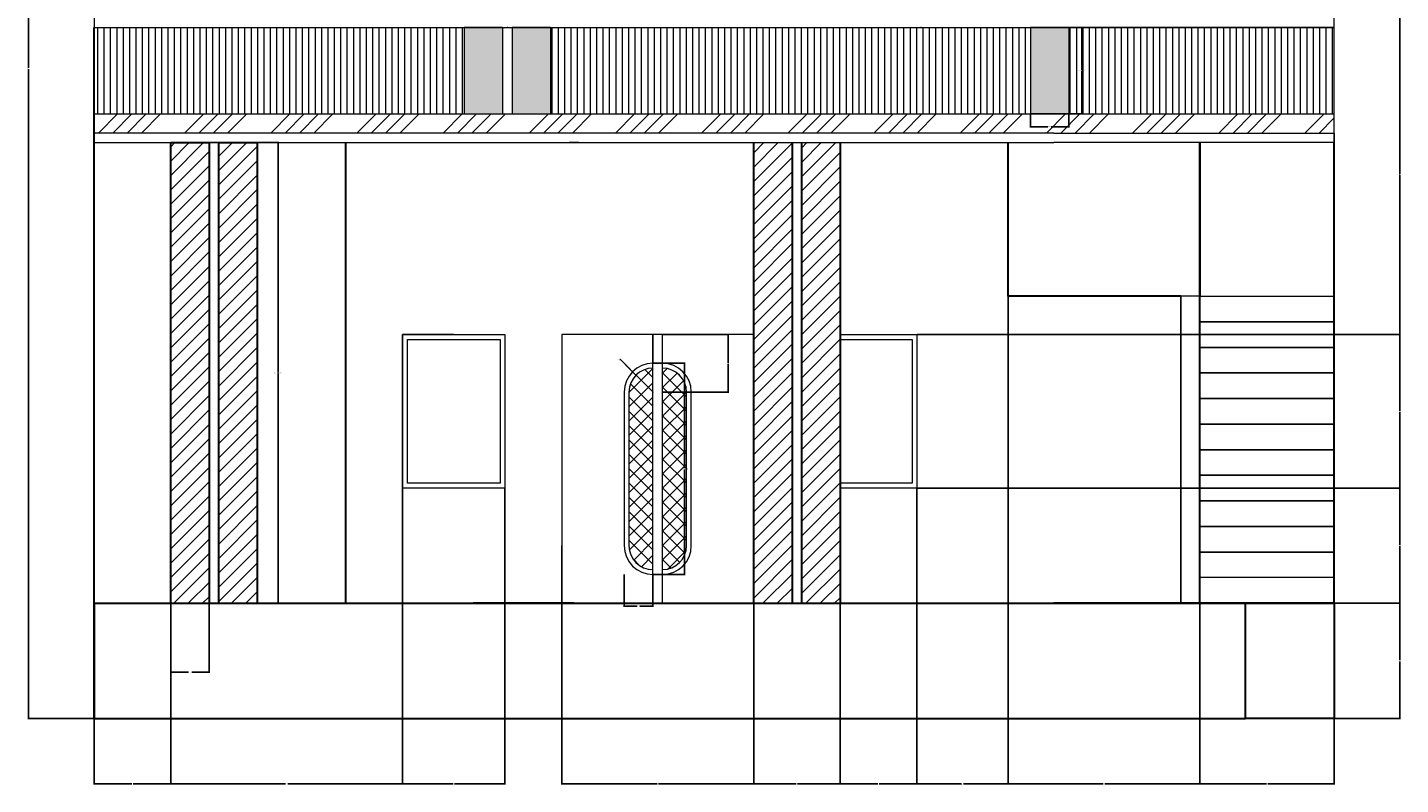
# Model space of a CAD drawing. Units: inches. Extents: x 2156 to 3149, y 1513 to 2286.
# Tile 4 of 5: x 2720 to 3149, y 1838 to 2075. Entities that reach past the tile are written whole.
import ezdxf

# ---------------------------------------------------------------- set-up
doc = ezdxf.new("R2010")
doc.units = ezdxf.units.IN
for name, color, linetype, lineweight in [('A-ANNO-DIMS', 2, 'Continuous', 18), ('A-CONS', 8, 'Continuous', 9), ('A-ELEV', 7, 'Continuous', 30), ('A-ELEV-BASE', 7, 'Continuous', 30), ('A-ELEV-COLS', 7, 'Continuous', 30), ('A-ELEV-COLS-PATT', 8, 'Continuous', 13), ('A-ELEV-DOOR', 3, 'Continuous', 20), ('A-ELEV-DOOR-PATT', 8, 'Continuous', 13), ('A-ELEV-GLAZ', 4, 'Continuous', 18), ('A-ELEV-PATT', 18, 'Continuous', 13), ('A-ELEV-STRS', 7, 'Continuous', 20), ('A-ELEV-TRIM', 7, 'Continuous', 20), ('A-ELEV-TRIM-PATT', 8, 'Continuous', 13)]:
    doc.layers.add(name, color=color, linetype=linetype, lineweight=lineweight)
doc.styles.get("Standard").update_dxf_attribs({"font": 'arial.ttf'})
doc.dimstyles.get("Standard").update_dxf_attribs({"dimtxt": 0.18, "dimasz": 0.18, "dimexe": 0.18, "dimexo": 0.0625, "dimgap": 0.09, "dimtad": 0, "dimtih": 1, "dimtoh": 1, "dimdec": 4, "dimzin": 0, "dimdsep": 46, "dimtxsty": 'Standard', "dimcen": 0.09, "dimadec": 0, "dimazin": 0, "dimtfac": 1, "dimtdec": 4, "dimtofl": 0, "dimtmove": 0, "dimatfit": 3, "dimfxl": 1, "dimtolj": 1, "dimtzin": 0, "dimarcsym": 0})

# ---------------------------------------------------------------- blocks, each defined once
blk = doc.blocks.new('ENTRY-DOOR-OVAL-TRIM')
for p, q in [((0, 57), (0, 9)), ((1.5, 57), (1.5, 9))]:
    blk.add_line(p, q)
for centre, radius, start, end in [((9, 57), 9, 90, 180), ((9, 57), 7.5, 90, 180), ((9, 9), 9, 180, 270), ((9, 9), 7.5, 180, 270)]:
    blk.add_arc(centre, radius, start, end)
blk = doc.blocks.new('FASCIA-PIER-12X27')
for p, q in [((12, 27), (0, 27)), ((0, 27), (0, 0)), ((12, 27), (12, 0))]:
    blk.add_line(p, q)
blk = doc.blocks.new('PORCH-PIER-12X144-ELEV')
for p, q in [((0, 0), (0, 144)), ((0, 144), (12, 144)), ((12, 144), (12, 0))]:
    blk.add_line(p, q)
blk = doc.blocks.new('*D13')
at = {"layer": 'A-ANNO-DIMS', "color": 0, "lineweight": -2, "transparency": 16777216}
for p, q in [((3045.59, 2074.71), (3049.76, 2074.71)), ((3049.58, 2074.53), (3049.58, 2061.39)), ((3049.58, 2047.89), (3049.58, 2061.03)), ((3045.59, 2047.71), (3049.76, 2047.71))]:
    blk.add_line(p, q, dxfattribs=at)
at = {"layer": 'A-ANNO-DIMS', "color": 0, "transparency": 16777216}
for points in [[(3049.55, 2074.53), (3049.61, 2074.53), (3049.58, 2074.71)], [(3049.55, 2047.89), (3049.61, 2047.89), (3049.58, 2047.71)]]:
    blk.add_solid(points, dxfattribs=at)
at = {"layer": 'Defpoints', "color": 0, "transparency": 16777216}
for p in [(3045.53, 2074.71), (3049.58, 2074.71), (3045.53, 2047.71)]:
    blk.add_point(p, dxfattribs=at)
at = {"layer": 'A-ANNO-DIMS', "color": 0, "transparency": 16777216, "insert": (3049.58, 2061.21), "char_height": 0.18, "attachment_point": 5}
blk.add_mtext('\\A1;FASCIA PIER 27 TYP.', dxfattribs=at)
blk = doc.blocks.new('*D14')
at = {"layer": 'A-ANNO-DIMS', "color": 0, "lineweight": -2, "transparency": 16777216}
for p, q in [((3033.53, 2047.65), (3033.53, 2043.48)), ((3045.53, 2047.65), (3045.53, 2043.48)), ((3033.71, 2043.66), (3039.01, 2043.66)), ((3045.35, 2043.66), (3040.05, 2043.66))]:
    blk.add_line(p, q, dxfattribs=at)
at = {"layer": 'A-ANNO-DIMS', "color": 0, "transparency": 16777216}
for points in [[(3033.71, 2043.69), (3033.71, 2043.63), (3033.53, 2043.66)], [(3045.35, 2043.69), (3045.35, 2043.63), (3045.53, 2043.66)]]:
    blk.add_solid(points, dxfattribs=at)
at = {"layer": 'Defpoints', "color": 0, "transparency": 16777216}
for p in [(3033.53, 2047.71), (3045.53, 2047.71), (3045.53, 2043.66)]:
    blk.add_point(p, dxfattribs=at)
at = {"layer": 'A-ANNO-DIMS', "color": 0, "transparency": 16777216, "insert": (3039.53, 2043.66), "char_height": 0.18, "attachment_point": 5}
blk.add_mtext('\\A1;12 TYP.', dxfattribs=at)
blk = doc.blocks.new('*D15')
at = {"layer": 'A-ANNO-DIMS', "color": 0, "lineweight": -2, "transparency": 16777216}
for p, q in [((2915.59, 1969.71), (2925.61, 1969.71)), ((2925.43, 1969.53), (2925.43, 1936.89)), ((2925.43, 1903.89), (2925.43, 1936.53)), ((2915.59, 1903.71), (2925.61, 1903.71))]:
    blk.add_line(p, q, dxfattribs=at)
at = {"layer": 'A-ANNO-DIMS', "color": 0, "transparency": 16777216}
for points in [[(2925.4, 1969.53), (2925.46, 1969.53), (2925.43, 1969.71)], [(2925.4, 1903.89), (2925.46, 1903.89), (2925.43, 1903.71)]]:
    blk.add_solid(points, dxfattribs=at)
at = {"layer": 'Defpoints', "color": 0, "transparency": 16777216}
for p in [(2915.53, 1969.71), (2925.43, 1969.71), (2915.53, 1903.71)]:
    blk.add_point(p, dxfattribs=at)
at = {"layer": 'A-ANNO-DIMS', "color": 0, "transparency": 16777216, "insert": (2925.43, 1936.71), "char_height": 0.18, "attachment_point": 5}
blk.add_mtext('\\A1;DOOR TRIM 66 TYP.', dxfattribs=at)
blk = doc.blocks.new('*D16')
at = {"layer": 'A-ANNO-DIMS', "color": 0, "lineweight": -2, "transparency": 16777216}
for p, q in [((2906.53, 1903.65), (2906.53, 1893.63)), ((2915.53, 1903.65), (2915.53, 1893.63)), ((2906.71, 1893.81), (2910.57, 1893.81)), ((2915.35, 1893.81), (2911.48, 1893.81))]:
    blk.add_line(p, q, dxfattribs=at)
at = {"layer": 'A-ANNO-DIMS', "color": 0, "transparency": 16777216}
for points in [[(2906.71, 1893.84), (2906.71, 1893.78), (2906.53, 1893.81)], [(2915.35, 1893.84), (2915.35, 1893.78), (2915.53, 1893.81)]]:
    blk.add_solid(points, dxfattribs=at)
at = {"layer": 'Defpoints', "color": 0, "transparency": 16777216}
for p in [(2906.53, 1903.71), (2915.53, 1903.71), (2915.53, 1893.81)]:
    blk.add_point(p, dxfattribs=at)
at = {"layer": 'A-ANNO-DIMS', "color": 0, "transparency": 16777216, "insert": (2911.03, 1893.81), "char_height": 0.18, "attachment_point": 5}
blk.add_mtext('\\A1;9 TYP.', dxfattribs=at)
blk = doc.blocks.new('*D17')
at = {"layer": 'A-ANNO-DIMS', "color": 0, "lineweight": -2, "transparency": 16777216}
for p, q in [((2776.88, 2038.71), (2798.6, 2038.71)), ((2798.42, 2038.53), (2798.42, 1966.89)), ((2798.42, 1894.89), (2798.42, 1966.53)), ((2776.88, 1894.71), (2798.6, 1894.71))]:
    blk.add_line(p, q, dxfattribs=at)
at = {"layer": 'A-ANNO-DIMS', "color": 0, "transparency": 16777216}
for points in [[(2798.39, 2038.53), (2798.45, 2038.53), (2798.42, 2038.71)], [(2798.39, 1894.89), (2798.45, 1894.89), (2798.42, 1894.71)]]:
    blk.add_solid(points, dxfattribs=at)
at = {"layer": 'Defpoints', "color": 0, "transparency": 16777216}
for p in [(2776.82, 2038.71), (2798.42, 2038.71), (2776.82, 1894.71)]:
    blk.add_point(p, dxfattribs=at)
at = {"layer": 'A-ANNO-DIMS', "color": 0, "transparency": 16777216, "insert": (2798.42, 1966.71), "char_height": 0.18, "attachment_point": 5}
blk.add_mtext('\\A1;PORCH PIER 144 TYP.', dxfattribs=at)
blk = doc.blocks.new('*D18')
at = {"layer": 'A-ANNO-DIMS', "color": 0, "lineweight": -2, "transparency": 16777216}
for p, q in [((2764.82, 1894.65), (2764.82, 1872.93)), ((2776.82, 1894.65), (2776.82, 1872.93)), ((2765, 1873.11), (2770.3, 1873.11)), ((2776.64, 1873.11), (2771.34, 1873.11))]:
    blk.add_line(p, q, dxfattribs=at)
at = {"layer": 'A-ANNO-DIMS', "color": 0, "transparency": 16777216}
for points in [[(2765, 1873.14), (2765, 1873.08), (2764.82, 1873.11)], [(2776.64, 1873.14), (2776.64, 1873.08), (2776.82, 1873.11)]]:
    blk.add_solid(points, dxfattribs=at)
at = {"layer": 'Defpoints', "color": 0, "transparency": 16777216}
for p in [(2764.82, 1894.71), (2776.82, 1894.71), (2776.82, 1873.11)]:
    blk.add_point(p, dxfattribs=at)
at = {"layer": 'A-ANNO-DIMS', "color": 0, "transparency": 16777216, "insert": (2770.82, 1873.11), "char_height": 0.18, "attachment_point": 5}
blk.add_mtext('\\A1;12 TYP.', dxfattribs=at)
blk = doc.blocks.new('*D46')
at = {"layer": 'A-ANNO-DIMS', "color": 0, "lineweight": -2, "transparency": 16777216}
for p, q in [((3071.46, 2265.09), (2720.14, 2265.09)), ((2720.32, 2264.91), (2720.32, 2062.08)), ((2720.32, 1858.89), (2720.32, 2061.72)), ((2740.75, 1858.71), (2720.14, 1858.71))]:
    blk.add_line(p, q, dxfattribs=at)
at = {"layer": 'A-ANNO-DIMS', "color": 0, "transparency": 16777216}
for points in [[(2720.29, 2264.91), (2720.35, 2264.91), (2720.32, 2265.09)], [(2720.29, 1858.89), (2720.35, 1858.89), (2720.32, 1858.71)]]:
    blk.add_solid(points, dxfattribs=at)
at = {"layer": 'Defpoints', "color": 0, "transparency": 16777216}
for p in [(2720.32, 2265.09), (3071.53, 2265.09), (2740.82, 1858.71)]:
    blk.add_point(p, dxfattribs=at)
at = {"layer": 'A-ANNO-DIMS', "color": 0, "transparency": 16777216, "insert": (2720.32, 2061.9), "char_height": 0.18, "attachment_point": 5}
blk.add_mtext('\\A1;406.4', dxfattribs=at)
blk = doc.blocks.new('*D48')
at = {"layer": 'A-ANNO-DIMS', "color": 0, "lineweight": -2, "transparency": 16777216}
for p, q in [((2918.59, 1978.71), (2939.21, 1978.71)), ((2939.03, 1978.53), (2939.03, 1969.89)), ((2939.03, 1960.89), (2939.03, 1969.53)), ((2918.59, 1960.71), (2939.21, 1960.71))]:
    blk.add_line(p, q, dxfattribs=at)
at = {"layer": 'A-ANNO-DIMS', "color": 0, "transparency": 16777216}
for points in [[(2939, 1978.53), (2939.06, 1978.53), (2939.03, 1978.71)], [(2939, 1960.89), (2939.06, 1960.89), (2939.03, 1960.71)]]:
    blk.add_solid(points, dxfattribs=at)
at = {"layer": 'Defpoints', "color": 0, "transparency": 16777216}
for p in [(2918.53, 1978.71), (2918.53, 1960.71), (2939.03, 1960.71)]:
    blk.add_point(p, dxfattribs=at)
at = {"layer": 'A-ANNO-DIMS', "color": 0, "transparency": 16777216, "insert": (2939.03, 1969.71), "char_height": 0.18, "attachment_point": 5}
blk.add_mtext('\\A1;18', dxfattribs=at)
blk = doc.blocks.new('*D51')
at = {"layer": 'A-ANNO-DIMS', "color": 0, "lineweight": -2, "transparency": 16777216}
for p, q in [((3128.59, 1894.71), (3149.21, 1894.71)), ((3149.03, 1894.53), (3149.03, 1876.89)), ((3149.03, 1858.89), (3149.03, 1876.53)), ((3128.59, 1858.71), (3149.21, 1858.71))]:
    blk.add_line(p, q, dxfattribs=at)
at = {"layer": 'A-ANNO-DIMS', "color": 0, "transparency": 16777216}
for points in [[(3149, 1894.53), (3149.06, 1894.53), (3149.03, 1894.71)], [(3149, 1858.89), (3149.06, 1858.89), (3149.03, 1858.71)]]:
    blk.add_solid(points, dxfattribs=at)
at = {"layer": 'Defpoints', "color": 0, "transparency": 16777216}
for p in [(3128.53, 1894.71), (3149.03, 1894.71), (3128.53, 1858.71)]:
    blk.add_point(p, dxfattribs=at)
at = {"layer": 'A-ANNO-DIMS', "color": 0, "transparency": 16777216, "insert": (3149.03, 1876.71), "char_height": 0.18, "attachment_point": 5}
blk.add_mtext('\\A1;36', dxfattribs=at)
blk = doc.blocks.new('*D52')
at = {"layer": 'A-ANNO-DIMS', "color": 0, "lineweight": -2, "transparency": 16777216}
for p, q in [((2998.09, 1930.71), (3149.21, 1930.71)), ((3149.03, 1930.53), (3149.03, 1912.89)), ((3149.03, 1894.89), (3149.03, 1912.53)), ((3128.59, 1894.71), (3149.21, 1894.71))]:
    blk.add_line(p, q, dxfattribs=at)
at = {"layer": 'A-ANNO-DIMS', "color": 0, "transparency": 16777216}
for points in [[(3149, 1930.53), (3149.06, 1930.53), (3149.03, 1930.71)], [(3149, 1894.89), (3149.06, 1894.89), (3149.03, 1894.71)]]:
    blk.add_solid(points, dxfattribs=at)
at = {"layer": 'Defpoints', "color": 0, "transparency": 16777216}
for p in [(2998.03, 1930.71), (3149.03, 1930.71), (3128.53, 1894.71)]:
    blk.add_point(p, dxfattribs=at)
at = {"layer": 'A-ANNO-DIMS', "color": 0, "transparency": 16777216, "insert": (3149.03, 1912.71), "char_height": 0.18, "attachment_point": 5}
blk.add_mtext('\\A1;36', dxfattribs=at)
blk = doc.blocks.new('*D53')
at = {"layer": 'A-ANNO-DIMS', "color": 0, "lineweight": -2, "transparency": 16777216}
for p, q in [((2998.09, 1978.71), (3149.21, 1978.71)), ((3149.03, 1978.53), (3149.03, 1954.89)), ((3149.03, 1930.89), (3149.03, 1954.53)), ((2998.09, 1930.71), (3149.21, 1930.71))]:
    blk.add_line(p, q, dxfattribs=at)
at = {"layer": 'A-ANNO-DIMS', "color": 0, "transparency": 16777216}
for points in [[(3149, 1978.53), (3149.06, 1978.53), (3149.03, 1978.71)], [(3149, 1930.89), (3149.06, 1930.89), (3149.03, 1930.71)]]:
    blk.add_solid(points, dxfattribs=at)
at = {"layer": 'Defpoints', "color": 0, "transparency": 16777216}
for p in [(2998.03, 1978.71), (3149.03, 1978.71), (2998.03, 1930.71)]:
    blk.add_point(p, dxfattribs=at)
at = {"layer": 'A-ANNO-DIMS', "color": 0, "transparency": 16777216, "insert": (3149.03, 1954.71), "char_height": 0.18, "attachment_point": 5}
blk.add_mtext('\\A1;48', dxfattribs=at)
blk = doc.blocks.new('*D54')
at = {"layer": 'A-ANNO-DIMS', "color": 0, "lineweight": -2, "transparency": 16777216}
for p, q in [((3128.59, 2078.71), (3149.21, 2078.71)), ((3149.03, 2078.53), (3149.03, 2028.89)), ((3149.03, 1978.89), (3149.03, 2028.53)), ((2998.09, 1978.71), (3149.21, 1978.71))]:
    blk.add_line(p, q, dxfattribs=at)
at = {"layer": 'A-ANNO-DIMS', "color": 0, "transparency": 16777216}
for points in [[(3149, 2078.53), (3149.06, 2078.53), (3149.03, 2078.71)], [(3149, 1978.89), (3149.06, 1978.89), (3149.03, 1978.71)]]:
    blk.add_solid(points, dxfattribs=at)
at = {"layer": 'Defpoints', "color": 0, "transparency": 16777216}
for p in [(3128.53, 2078.71), (3149.03, 2078.71), (2998.03, 1978.71)]:
    blk.add_point(p, dxfattribs=at)
at = {"layer": 'A-ANNO-DIMS', "color": 0, "transparency": 16777216, "insert": (3149.03, 2028.71), "char_height": 0.18, "attachment_point": 5}
blk.add_mtext('\\A1;100', dxfattribs=at)
blk = doc.blocks.new('*D58')
at = {"layer": 'A-ANNO-DIMS', "color": 0, "lineweight": -2, "transparency": 16777216}
for p, q in [((2764.82, 1894.65), (2764.82, 1838.03)), ((2740.82, 1858.65), (2740.82, 1838.03)), ((2741, 1838.21), (2752.6, 1838.21)), ((2764.64, 1838.21), (2753.04, 1838.21))]:
    blk.add_line(p, q, dxfattribs=at)
at = {"layer": 'A-ANNO-DIMS', "color": 0, "transparency": 16777216}
for points in [[(2741, 1838.24), (2741, 1838.18), (2740.82, 1838.21)], [(2764.64, 1838.24), (2764.64, 1838.18), (2764.82, 1838.21)]]:
    blk.add_solid(points, dxfattribs=at)
at = {"layer": 'Defpoints', "color": 0, "transparency": 16777216}
for p in [(2764.82, 1894.71), (2740.82, 1858.71), (2764.82, 1838.21)]:
    blk.add_point(p, dxfattribs=at)
at = {"layer": 'A-ANNO-DIMS', "color": 0, "transparency": 16777216, "insert": (2752.82, 1838.21), "char_height": 0.18, "attachment_point": 5}
blk.add_mtext('\\A1;24', dxfattribs=at)
blk = doc.blocks.new('*D59')
at = {"layer": 'A-ANNO-DIMS', "color": 0, "lineweight": -2, "transparency": 16777216}
for p, q in [((2837.28, 1930.65), (2837.28, 1838.03)), ((2764.82, 1894.65), (2764.82, 1838.03)), ((2765, 1838.21), (2800.65, 1838.21)), ((2837.1, 1838.21), (2801.44, 1838.21))]:
    blk.add_line(p, q, dxfattribs=at)
at = {"layer": 'A-ANNO-DIMS', "color": 0, "transparency": 16777216}
for points in [[(2765, 1838.24), (2765, 1838.18), (2764.82, 1838.21)], [(2837.1, 1838.24), (2837.1, 1838.18), (2837.28, 1838.21)]]:
    blk.add_solid(points, dxfattribs=at)
at = {"layer": 'Defpoints', "color": 0, "transparency": 16777216}
for p in [(2837.28, 1930.71), (2764.82, 1894.71), (2837.28, 1838.21)]:
    blk.add_point(p, dxfattribs=at)
at = {"layer": 'A-ANNO-DIMS', "color": 0, "transparency": 16777216, "insert": (2801.05, 1838.21), "char_height": 0.18, "attachment_point": 5}
blk.add_mtext('\\A1;72.46', dxfattribs=at)
blk = doc.blocks.new('*D60')
at = {"layer": 'A-ANNO-DIMS', "color": 0, "lineweight": -2, "transparency": 16777216}
for p, q in [((2837.28, 1930.65), (2837.28, 1838.03)), ((2869.28, 1930.65), (2869.28, 1838.03)), ((2837.46, 1838.21), (2853.06, 1838.21)), ((2869.1, 1838.21), (2853.49, 1838.21))]:
    blk.add_line(p, q, dxfattribs=at)
at = {"layer": 'A-ANNO-DIMS', "color": 0, "transparency": 16777216}
for points in [[(2837.46, 1838.24), (2837.46, 1838.18), (2837.28, 1838.21)], [(2869.1, 1838.24), (2869.1, 1838.18), (2869.28, 1838.21)]]:
    blk.add_solid(points, dxfattribs=at)
at = {"layer": 'Defpoints', "color": 0, "transparency": 16777216}
for p in [(2837.28, 1930.71), (2869.28, 1930.71), (2869.28, 1838.21)]:
    blk.add_point(p, dxfattribs=at)
at = {"layer": 'A-ANNO-DIMS', "color": 0, "transparency": 16777216, "insert": (2853.28, 1838.21), "char_height": 0.18, "attachment_point": 5}
blk.add_mtext('\\A1;32', dxfattribs=at)
blk = doc.blocks.new('*D61')
at = {"layer": 'A-ANNO-DIMS', "color": 0, "lineweight": -2, "transparency": 16777216}
for p, q in [((2887.03, 1894.65), (2887.03, 1838.03)), ((2947.03, 1894.65), (2947.03, 1838.03)), ((2887.21, 1838.21), (2916.81, 1838.21)), ((2946.85, 1838.21), (2917.25, 1838.21))]:
    blk.add_line(p, q, dxfattribs=at)
at = {"layer": 'A-ANNO-DIMS', "color": 0, "transparency": 16777216}
for points in [[(2887.21, 1838.24), (2887.21, 1838.18), (2887.03, 1838.21)], [(2946.85, 1838.24), (2946.85, 1838.18), (2947.03, 1838.21)]]:
    blk.add_solid(points, dxfattribs=at)
at = {"layer": 'Defpoints', "color": 0, "transparency": 16777216}
for p in [(2887.03, 1894.71), (2947.03, 1894.71), (2947.03, 1838.21)]:
    blk.add_point(p, dxfattribs=at)
at = {"layer": 'A-ANNO-DIMS', "color": 0, "transparency": 16777216, "insert": (2917.03, 1838.21), "char_height": 0.18, "attachment_point": 5}
blk.add_mtext('\\A1;60', dxfattribs=at)
blk = doc.blocks.new('*D62')
at = {"layer": 'A-ANNO-DIMS', "color": 0, "lineweight": -2, "transparency": 16777216}
for p, q in [((2974.03, 1930.65), (2974.03, 1838.03)), ((2947.03, 1894.65), (2947.03, 1838.03)), ((2947.21, 1838.21), (2960.31, 1838.21)), ((2973.85, 1838.21), (2960.75, 1838.21))]:
    blk.add_line(p, q, dxfattribs=at)
at = {"layer": 'A-ANNO-DIMS', "color": 0, "transparency": 16777216}
for points in [[(2947.21, 1838.24), (2947.21, 1838.18), (2947.03, 1838.21)], [(2973.85, 1838.24), (2973.85, 1838.18), (2974.03, 1838.21)]]:
    blk.add_solid(points, dxfattribs=at)
at = {"layer": 'Defpoints', "color": 0, "transparency": 16777216}
for p in [(2974.03, 1930.71), (2947.03, 1894.71), (2974.03, 1838.21)]:
    blk.add_point(p, dxfattribs=at)
at = {"layer": 'A-ANNO-DIMS', "color": 0, "transparency": 16777216, "insert": (2960.53, 1838.21), "char_height": 0.18, "attachment_point": 5}
blk.add_mtext('\\A1;27', dxfattribs=at)
blk = doc.blocks.new('*D63')
at = {"layer": 'A-ANNO-DIMS', "color": 0, "lineweight": -2, "transparency": 16777216}
for p, q in [((2974.03, 1930.65), (2974.03, 1838.03)), ((2998.03, 1930.65), (2998.03, 1838.03)), ((2974.21, 1838.21), (2985.81, 1838.21)), ((2997.85, 1838.21), (2986.25, 1838.21))]:
    blk.add_line(p, q, dxfattribs=at)
at = {"layer": 'A-ANNO-DIMS', "color": 0, "transparency": 16777216}
for points in [[(2974.21, 1838.24), (2974.21, 1838.18), (2974.03, 1838.21)], [(2997.85, 1838.24), (2997.85, 1838.18), (2998.03, 1838.21)]]:
    blk.add_solid(points, dxfattribs=at)
at = {"layer": 'Defpoints', "color": 0, "transparency": 16777216}
for p in [(2974.03, 1930.71), (2998.03, 1930.71), (2998.03, 1838.21)]:
    blk.add_point(p, dxfattribs=at)
at = {"layer": 'A-ANNO-DIMS', "color": 0, "transparency": 16777216, "insert": (2986.03, 1838.21), "char_height": 0.18, "attachment_point": 5}
blk.add_mtext('\\A1;24', dxfattribs=at)
blk = doc.blocks.new('*D64')
at = {"layer": 'A-ANNO-DIMS', "color": 0, "lineweight": -2, "transparency": 16777216}
for p, q in [((3026.53, 1990.65), (3026.53, 1838.03)), ((2998.03, 1930.65), (2998.03, 1838.03)), ((2998.21, 1838.21), (3011.95, 1838.21)), ((3026.35, 1838.21), (3012.6, 1838.21))]:
    blk.add_line(p, q, dxfattribs=at)
at = {"layer": 'A-ANNO-DIMS', "color": 0, "transparency": 16777216}
for points in [[(2998.21, 1838.24), (2998.21, 1838.18), (2998.03, 1838.21)], [(3026.35, 1838.24), (3026.35, 1838.18), (3026.53, 1838.21)]]:
    blk.add_solid(points, dxfattribs=at)
at = {"layer": 'Defpoints', "color": 0, "transparency": 16777216}
for p in [(3026.53, 1990.71), (2998.03, 1930.71), (3026.53, 1838.21)]:
    blk.add_point(p, dxfattribs=at)
at = {"layer": 'A-ANNO-DIMS', "color": 0, "transparency": 16777216, "insert": (3012.28, 1838.21), "char_height": 0.18, "attachment_point": 5}
blk.add_mtext('\\A1;28.5', dxfattribs=at)
blk = doc.blocks.new('*D65')
at = {"layer": 'A-ANNO-DIMS', "color": 0, "lineweight": -2, "transparency": 16777216}
for p, q in [((3026.53, 1990.65), (3026.53, 1838.03)), ((3086.53, 1894.65), (3086.53, 1838.03)), ((3026.71, 1838.21), (3056.31, 1838.21)), ((3086.35, 1838.21), (3056.75, 1838.21))]:
    blk.add_line(p, q, dxfattribs=at)
at = {"layer": 'A-ANNO-DIMS', "color": 0, "transparency": 16777216}
for points in [[(3026.71, 1838.24), (3026.71, 1838.18), (3026.53, 1838.21)], [(3086.35, 1838.24), (3086.35, 1838.18), (3086.53, 1838.21)]]:
    blk.add_solid(points, dxfattribs=at)
at = {"layer": 'Defpoints', "color": 0, "transparency": 16777216}
for p in [(3026.53, 1990.71), (3086.53, 1894.71), (3086.53, 1838.21)]:
    blk.add_point(p, dxfattribs=at)
at = {"layer": 'A-ANNO-DIMS', "color": 0, "transparency": 16777216, "insert": (3056.53, 1838.21), "char_height": 0.18, "attachment_point": 5}
blk.add_mtext('\\A1;60', dxfattribs=at)
blk = doc.blocks.new('*D66')
at = {"layer": 'A-ANNO-DIMS', "color": 0, "lineweight": -2, "transparency": 16777216}
for p, q in [((3086.53, 1894.65), (3086.53, 1838.03)), ((3128.53, 1858.65), (3128.53, 1838.03)), ((3086.71, 1838.21), (3107.3, 1838.21)), ((3128.35, 1838.21), (3107.75, 1838.21))]:
    blk.add_line(p, q, dxfattribs=at)
at = {"layer": 'A-ANNO-DIMS', "color": 0, "transparency": 16777216}
for points in [[(3086.71, 1838.24), (3086.71, 1838.18), (3086.53, 1838.21)], [(3128.35, 1838.24), (3128.35, 1838.18), (3128.53, 1838.21)]]:
    blk.add_solid(points, dxfattribs=at)
at = {"layer": 'Defpoints', "color": 0, "transparency": 16777216}
for p in [(3086.53, 1894.71), (3128.53, 1858.71), (3128.53, 1838.21)]:
    blk.add_point(p, dxfattribs=at)
at = {"layer": 'A-ANNO-DIMS', "color": 0, "transparency": 16777216, "insert": (3107.53, 1838.21), "char_height": 0.18, "attachment_point": 5}
blk.add_mtext('\\A1;42', dxfattribs=at)
blk = doc.blocks.new('*D88')
at = {"layer": 'A-ANNO-DIMS', "color": 0, "lineweight": -2, "transparency": 16777216}
for p, q in [((2905.16, 1970.89), (2905.34, 1970.89)), ((2905.34, 1970.89), (2909.03, 1967.2)), ((2915.44, 1960.71), (2915.62, 1960.71)), ((2915.53, 1960.62), (2915.53, 1960.8))]:
    blk.add_line(p, q, dxfattribs=at)
at = {"layer": 'A-ANNO-DIMS', "color": 0, "transparency": 16777216}
blk.add_solid([(2909.06, 1967.22), (2909.01, 1967.18), (2909.16, 1967.07)], dxfattribs=at)
at = {"layer": 'Defpoints', "color": 0, "transparency": 16777216}
for p in [(2909.16, 1967.07), (2915.53, 1960.71)]:
    blk.add_point(p, dxfattribs=at)
at = {"layer": 'A-ANNO-DIMS', "color": 0, "transparency": 16777216, "insert": (2904.73, 1970.89), "char_height": 0.18, "attachment_point": 5}
blk.add_mtext('\\A1;4X R9', dxfattribs=at)
blk = doc.blocks.new('*D89')
at = {"layer": 'A-ANNO-DIMS', "color": 0, "lineweight": -2, "transparency": 16777216}
for p, q in [((2906.86, 1969.19), (2907.04, 1969.19)), ((2907.04, 1969.19), (2910.1, 1966.14)), ((2915.44, 1960.71), (2915.62, 1960.71)), ((2915.53, 1960.62), (2915.53, 1960.8))]:
    blk.add_line(p, q, dxfattribs=at)
at = {"layer": 'A-ANNO-DIMS', "color": 0, "transparency": 16777216}
blk.add_solid([(2910.12, 1966.16), (2910.07, 1966.12), (2910.22, 1966.01)], dxfattribs=at)
at = {"layer": 'Defpoints', "color": 0, "transparency": 16777216}
for p in [(2910.22, 1966.01), (2915.53, 1960.71)]:
    blk.add_point(p, dxfattribs=at)
at = {"layer": 'A-ANNO-DIMS', "color": 0, "transparency": 16777216, "insert": (2906.32, 1969.19), "char_height": 0.18, "attachment_point": 5}
blk.add_mtext('\\A1;4X R7.5', dxfattribs=at)

msp = doc.modelspace()

# ---------------------------------------------------------------- hatches: boundary and pattern name
at = {"layer": 'A-ELEV-COLS-PATT'}
h = msp.add_hatch(dxfattribs=at)
h.set_pattern_fill('ANSI31', color=256)
h.paths.add_polyline_path([(2776.816, 2038.708), (2764.816, 2038.708), (2764.816, 1894.708), (2776.816, 1894.708)])
h.paths.add_polyline_path([(2791.816, 2038.708), (2779.816, 2038.708), (2779.816, 1894.708), (2791.816, 1894.708)])
h.paths.add_polyline_path([(2959.026, 2038.708), (2947.026, 2038.708), (2947.026, 1894.708), (2959.026, 1894.708)])
h.paths.add_polyline_path([(2974.026, 2038.708), (2962.026, 2038.708), (2962.026, 1894.708), (2974.026, 1894.708)])
at = {"layer": 'A-ELEV-DOOR-PATT'}
h = msp.add_hatch(dxfattribs=at)
h.set_pattern_fill('ANSI37', color=256)
h.paths.add_polyline_path([(2915.526, 1968.208, 0.4142136), (2908.026, 1960.708), (2908.026, 1912.708, 0.4142136), (2915.526, 1905.208)])
h.paths.add_polyline_path([(2926.026, 1960.708, 0.4142136), (2918.526, 1968.208), (2918.526, 1905.208, 0.4142136), (2926.026, 1912.708)])
at = {"layer": 'A-ELEV-PATT'}
h = msp.add_hatch(color=256, dxfattribs=at)
h.dxf.hatch_style = 1
h.paths.add_polyline_path([(2868.553, 2074.708), (2856.553, 2074.708), (2856.553, 2047.708), (2868.553, 2047.708)])
h = msp.add_hatch(color=256, dxfattribs=at)
h.dxf.hatch_style = 1
h.paths.add_polyline_path([(2883.553, 2074.708), (2871.553, 2074.708), (2871.553, 2047.708), (2883.553, 2047.708)])
h.paths.add_polyline_path([(3045.526, 2074.708), (3033.526, 2074.708), (3033.526, 2047.708), (3045.526, 2047.708)])
at = {"layer": 'A-ELEV-TRIM-PATT'}
h = msp.add_hatch(dxfattribs=at)
h.set_pattern_fill('ANSI31', color=256, scale=0.629921, angle=45, style=0)
h.paths.add_polyline_path([(2740.816, 2047.708), (2856.553, 2047.708), (2856.553, 2074.708), (2740.816, 2074.708)])
h = msp.add_hatch(dxfattribs=at)
h.set_pattern_fill('ANSI31', color=256, scale=0.629921, angle=45, style=0)
h.paths.add_polyline_path([(2883.553, 2047.708), (3033.526, 2047.708), (3033.526, 2074.708), (2883.553, 2074.708)])
h = msp.add_hatch(dxfattribs=at)
h.set_pattern_fill('ANSI31', color=256, scale=0.629921, angle=45, style=0)
h.paths.add_polyline_path([(3045.526, 2047.708), (3128.526, 2047.708), (3128.526, 2074.708), (3045.526, 2074.708)])
h = msp.add_hatch(dxfattribs=at)
h.set_pattern_fill('ANSI34', color=256)
h.paths.add_polyline_path([(3128.526, 2047.708), (2740.816, 2047.708), (2740.816, 2041.708), (3040.816, 2041.708), (3128.526, 2041.708)])

# ---------------------------------------------------------------- linework, layer by layer
at = {"layer": 'A-CONS'}
for p in [(2870.053, 2074.708), (2999.289, 2074.708), (3128.526, 1982.708), (3128.526, 1974.708), (3128.526, 1966.708), (3128.526, 1958.708), (3128.526, 1950.708), (3128.526, 1942.708), (3128.526, 1934.708), (3128.526, 1926.708), (3128.526, 1918.708), (3128.526, 1910.708), (3128.526, 1902.708)]:
    msp.add_point(p, dxfattribs=at)
at = {"layer": 'A-ELEV'}
for p, q in [((2740.816, 1894.708), (2740.816, 2074.708)), ((2740.816, 1894.708), (2740.816, 2038.708)), ((2819.526, 1894.708), (2819.526, 2038.708)), ((3026.526, 1990.708), (3026.526, 2038.708)), ((3086.526, 1894.708), (3086.526, 2038.708)), ((3086.526, 2038.708), (3086.526, 1990.708)), ((3128.526, 1894.708), (3128.526, 2038.708)), ((3080.526, 1990.708), (3026.526, 1990.708))]:
    msp.add_line(p, q, dxfattribs=at)
at = {"layer": 'A-ELEV-BASE'}
for p, q in [((2740.816, 1894.708), (2740.816, 1858.708)), ((2740.816, 1858.708), (2740.816, 1894.708)), ((2740.816, 1894.708), (2764.816, 1894.708)), ((2791.816, 1894.708), (2890.816, 1894.708)), ((2791.816, 1894.708), (2829.316, 1894.708)), ((2791.816, 1894.708), (2819.526, 1894.708)), ((2819.526, 1894.708), (3128.526, 1894.708)), ((2829.316, 1894.708), (2889.316, 1894.708)), ((2889.316, 1894.708), (2859.316, 1894.708)), ((2889.316, 1894.708), (2877.316, 1894.708)), ((2890.816, 1894.708), (2889.316, 1894.708)), ((2889.316, 1894.708), (2892.316, 1894.708)), ((3100.816, 1894.708), (3040.816, 1894.708)), ((3128.526, 1894.708), (3086.526, 1894.708)), ((3100.816, 1858.708), (3100.816, 1894.708)), ((3128.526, 1894.708), (3128.526, 1858.708)), ((2740.816, 1858.708), (3040.816, 1858.708)), ((3040.816, 1858.708), (3100.816, 1858.708)), ((3128.526, 1858.708), (3100.816, 1858.708))]:
    msp.add_line(p, q, dxfattribs=at)
at = {"layer": 'A-ELEV-COLS'}
for p, q in [((2947.026, 1894.708), (2947.026, 2038.708)), ((2959.026, 2038.708), (2959.026, 1894.708)), ((2962.026, 1894.708), (2962.026, 2038.708)), ((2974.026, 2038.708), (2974.026, 1894.708)), ((2764.816, 1894.708), (2791.816, 1894.708)), ((2776.816, 1894.708), (2779.816, 1894.708))]:
    msp.add_line(p, q, dxfattribs=at)
at = {"layer": 'A-ELEV-DOOR'}
for p, q in [((2899.026, 1978.708), (2887.026, 1978.708)), ((2887.026, 1978.708), (2887.026, 1894.708)), ((2887.026, 1978.708), (2887.026, 1960.708)), ((2947.026, 1978.708), (2899.026, 1978.708)), ((2915.526, 1894.708), (2915.526, 1978.708)), ((2915.526, 1978.708), (2915.526, 1969.708)), ((2918.526, 1894.708), (2918.526, 1978.708)), ((2918.526, 1969.708), (2918.526, 1978.708)), ((2947.026, 1894.708), (2947.026, 1978.708)), ((2887.026, 1894.708), (2887.026, 1912.708)), ((2915.526, 1894.708), (2915.526, 1903.708))]:
    msp.add_line(p, q, dxfattribs=at)
at = {"layer": 'A-ELEV-GLAZ'}
for p, q in [((2853.276, 1978.708), (2837.276, 1978.708)), ((2837.276, 1978.708), (2837.276, 1930.708)), ((2837.276, 1930.708), (2837.276, 1978.708)), ((2837.276, 1978.708), (2853.276, 1978.708)), ((2838.776, 1932.208), (2838.776, 1977.208)), ((2838.776, 1977.208), (2853.276, 1977.208)), ((2853.276, 1978.708), (2869.276, 1978.708)), ((2853.276, 1977.208), (2867.776, 1977.208)), ((2867.776, 1977.208), (2867.776, 1932.208)), ((2869.276, 1978.708), (2869.276, 1930.708)), ((2974.026, 1978.708), (2998.026, 1978.708)), ((2974.026, 1977.208), (2996.526, 1977.208)), ((2996.526, 1977.208), (2996.526, 1932.208)), ((2998.026, 1978.708), (2998.026, 1930.708)), ((2867.776, 1932.208), (2838.776, 1932.208)), ((2996.526, 1932.208), (2974.026, 1932.208)), ((2869.276, 1930.708), (2837.276, 1930.708)), ((2998.026, 1930.708), (2974.026, 1930.708))]:
    msp.add_line(p, q, dxfattribs=at)
at = {"layer": 'A-ELEV-STRS'}
for p, q in [((3086.526, 1990.708), (3080.526, 1990.708)), ((3080.526, 1990.708), (3080.526, 1894.708)), ((3080.526, 1894.708), (3080.526, 1990.708)), ((3086.526, 1990.708), (3128.526, 1990.708)), ((3128.526, 1990.708), (3128.526, 1894.708)), ((3128.526, 1982.708), (3086.526, 1982.708)), ((3086.526, 1982.708), (3128.526, 1982.708)), ((3128.526, 1982.708), (3128.526, 1974.708)), ((3128.526, 1974.708), (3086.526, 1974.708)), ((3086.526, 1974.708), (3128.526, 1974.708)), ((3128.526, 1974.708), (3128.526, 1966.708)), ((3128.526, 1966.708), (3086.526, 1966.708)), ((3086.526, 1966.708), (3128.526, 1966.708)), ((3128.526, 1966.708), (3128.526, 1958.708)), ((3128.526, 1958.708), (3086.526, 1958.708)), ((3086.526, 1958.708), (3128.526, 1958.708)), ((3128.526, 1958.708), (3128.526, 1950.708)), ((3128.526, 1950.708), (3086.526, 1950.708)), ((3086.526, 1950.708), (3128.526, 1950.708)), ((3128.526, 1950.708), (3128.526, 1942.708)), ((3128.526, 1942.708), (3086.526, 1942.708)), ((3086.526, 1942.708), (3128.526, 1942.708)), ((3128.526, 1942.708), (3128.526, 1934.708)), ((3128.526, 1934.708), (3086.526, 1934.708)), ((3086.526, 1934.708), (3128.526, 1934.708)), ((3128.526, 1934.708), (3128.526, 1926.708)), ((3128.526, 1926.708), (3086.526, 1926.708)), ((3086.526, 1926.708), (3128.526, 1926.708)), ((3128.526, 1926.708), (3128.526, 1918.708)), ((3128.526, 1918.708), (3086.526, 1918.708)), ((3086.526, 1918.708), (3128.526, 1918.708)), ((3128.526, 1918.708), (3128.526, 1910.708)), ((3128.526, 1910.708), (3086.526, 1910.708)), ((3086.526, 1910.708), (3128.526, 1910.708)), ((3128.526, 1910.708), (3128.526, 1902.708)), ((3128.526, 1902.708), (3086.526, 1902.708))]:
    msp.add_line(p, q, dxfattribs=at)
at = {"layer": 'A-ELEV-TRIM'}
for p, q in [((2740.816, 2078.708), (2740.816, 2074.708)), ((3128.526, 2074.708), (3128.526, 2078.708)), ((2740.816, 2074.708), (3040.816, 2074.708)), ((2740.816, 2074.708), (3128.526, 2074.708)), ((3128.526, 2074.708), (3040.816, 2074.708)), ((3128.526, 2038.708), (3128.526, 2074.708)), ((3128.526, 2047.708), (3128.526, 2074.708)), ((2740.816, 2041.708), (2740.816, 2047.708)), ((2740.816, 2047.708), (3128.526, 2047.708)), ((3045.526, 2047.708), (3033.526, 2047.708)), ((3040.816, 2041.708), (2740.816, 2041.708)), ((3040.816, 2041.708), (3128.526, 2041.708)), ((3128.526, 2041.708), (3128.526, 2038.708)), ((2740.816, 2038.708), (3040.816, 2038.708)), ((2877.316, 2038.708), (2892.316, 2038.708)), ((2892.316, 2038.708), (2889.316, 2038.708)), ((2892.316, 2038.708), (2904.316, 2038.708)), ((3128.526, 2038.708), (3040.816, 2038.708))]:
    msp.add_line(p, q, dxfattribs=at)

# ---------------------------------------------------------------- block references
at = {"layer": 'A-ELEV-COLS'}
for p in [(2764.816, 1894.708), (2779.816, 1894.708)]:
    msp.add_blockref('PORCH-PIER-12X144-ELEV', p, dxfattribs=at)
at = {"layer": 'A-ELEV-DOOR'}
msp.add_blockref('ENTRY-DOOR-OVAL-TRIM', (2906.526, 1903.708), dxfattribs=at)
at = {"layer": 'A-ELEV-DOOR', "rotation": 180}
msp.add_blockref('ENTRY-DOOR-OVAL-TRIM', (2927.526, 1969.708), dxfattribs=at)
at = {"layer": 'A-ELEV-TRIM'}
for p in [(2856.553, 2047.708), (2871.553, 2047.708), (3033.526, 2047.708)]:
    msp.add_blockref('FASCIA-PIER-12X27', p, dxfattribs=at)

# ---------------------------------------------------------------- dimensions: what is measured, and where the dimension line sits
at = {"layer": 'A-ANNO-DIMS'}
for base, p1, p2, angle, override, picture, middle in [((2720.316, 2265.094), (2740.816, 1858.708), (3071.526, 2265.094), 90, {"dimdec": 1, "dimlfac": 1, "dimrnd": 0, "dimzin": 0, "dimdsep": 46, "dimlunit": 2}, '*D46', (2720.316, 2061.901)), ((3149.026, 2078.708), (2998.026, 1978.708), (3128.526, 2078.708), 90, {"dimdec": 0, "dimlfac": 1, "dimrnd": 0, "dimzin": 0, "dimdsep": 46, "dimlunit": 2}, '*D54', (3149.026, 2028.708)), ((2939.026, 1960.708), (2918.526, 1978.708), (2918.526, 1960.708), 270, {"dimdec": 0, "dimlfac": 1, "dimrnd": 0, "dimzin": 0, "dimdsep": 46, "dimlunit": 2}, '*D48', (2939.026, 1969.708)), ((3149.026, 1978.708), (2998.026, 1930.708), (2998.026, 1978.708), 90, {"dimdec": 0, "dimlfac": 1, "dimrnd": 0, "dimzin": 0, "dimdsep": 46, "dimlunit": 2}, '*D53', (3149.026, 1954.708)), ((3149.026, 1930.708), (3128.526, 1894.708), (2998.026, 1930.708), 90, {"dimdec": 0, "dimlfac": 1, "dimrnd": 0, "dimzin": 0, "dimdsep": 46, "dimlunit": 2}, '*D52', (3149.026, 1912.708)), ((3149.026, 1894.708), (3128.526, 1858.708), (3128.526, 1894.708), 90, {"dimdec": 0, "dimlfac": 1, "dimrnd": 0, "dimzin": 0, "dimdsep": 46, "dimlunit": 2}, '*D51', (3149.026, 1876.708))]:
    dim = msp.add_linear_dim(base=base, p1=p1, p2=p2, angle=angle, dimstyle='Standard', override=override, dxfattribs=at)
    dim.commit()
    dim.dimension.update_dxf_attribs({"geometry": picture, "text_midpoint": middle})
for base, p1, p2, text, picture, middle in [((3049.576, 2074.708), (3045.526, 2047.708), (3045.526, 2074.708), 'FASCIA PIER <> TYP.', '*D13', (3049.576, 2061.208)), ((2798.416, 2038.708), (2776.816, 1894.708), (2776.816, 2038.708), 'PORCH PIER <> TYP.', '*D17', (2798.416, 1966.708)), ((2925.426, 1969.708), (2915.526, 1903.708), (2915.526, 1969.708), 'DOOR TRIM <> TYP.', '*D15', (2925.426, 1936.708))]:
    dim = msp.add_linear_dim(base=base, p1=p1, p2=p2, angle=90, text=text, dimstyle='Standard', override={"dimdec": 0, "dimlfac": 1, "dimrnd": 0, "dimzin": 0, "dimdsep": 46, "dimlunit": 2}, dxfattribs=at)
    dim.commit()
    dim.dimension.update_dxf_attribs({"geometry": picture, "text_midpoint": middle})
for base, p1, p2, picture, middle in [((3045.526, 2043.658), (3033.526, 2047.708), (3045.526, 2047.708), '*D14', (3039.526, 2043.658)), ((2915.526, 1893.808), (2906.526, 1903.708), (2915.526, 1903.708), '*D16', (2911.026, 1893.808)), ((2776.816, 1873.108), (2764.816, 1894.708), (2776.816, 1894.708), '*D18', (2770.816, 1873.108))]:
    dim = msp.add_linear_dim(base=base, p1=p1, p2=p2, text='<> TYP.', dimstyle='Standard', override={"dimdec": 0, "dimlfac": 1, "dimrnd": 0, "dimzin": 0, "dimdsep": 46, "dimlunit": 2}, dxfattribs=at)
    dim.commit()
    dim.dimension.update_dxf_attribs({"geometry": picture, "text_midpoint": middle})
for base, p1, p2, override, picture, middle in [((3026.526, 1838.208), (2998.026, 1930.708), (3026.526, 1990.708), {"dimdec": 1, "dimlfac": 1, "dimrnd": 0, "dimzin": 0, "dimdsep": 46, "dimlunit": 2}, '*D64', (3012.276, 1838.208)), ((3086.526, 1838.208), (3026.526, 1990.708), (3086.526, 1894.708), {"dimdec": 0, "dimlfac": 1, "dimrnd": 0, "dimzin": 0, "dimdsep": 46, "dimlunit": 2}, '*D65', (3056.526, 1838.208)), ((2837.276, 1838.208), (2764.816, 1894.708), (2837.276, 1930.708), {"dimdec": 2, "dimlfac": 1, "dimrnd": 0, "dimzin": 0, "dimdsep": 46, "dimlunit": 2}, '*D59', (2801.046, 1838.208)), ((2869.276, 1838.208), (2837.276, 1930.708), (2869.276, 1930.708), {"dimdec": 0, "dimlfac": 1, "dimrnd": 0, "dimzin": 0, "dimdsep": 46, "dimlunit": 2}, '*D60', (2853.276, 1838.208)), ((2974.026, 1838.208), (2947.026, 1894.708), (2974.026, 1930.708), {"dimdec": 0, "dimlfac": 1, "dimrnd": 0, "dimzin": 0, "dimdsep": 46, "dimlunit": 2}, '*D62', (2960.526, 1838.208)), ((2998.026, 1838.208), (2974.026, 1930.708), (2998.026, 1930.708), {"dimdec": 0, "dimlfac": 1, "dimrnd": 0, "dimzin": 0, "dimdsep": 46, "dimlunit": 2}, '*D63', (2986.026, 1838.208)), ((2764.816, 1838.208), (2740.816, 1858.708), (2764.816, 1894.708), {"dimdec": 0, "dimlfac": 1, "dimrnd": 0, "dimzin": 0, "dimdsep": 46, "dimlunit": 2}, '*D58', (2752.816, 1838.208)), ((2947.026, 1838.208), (2887.026, 1894.708), (2947.026, 1894.708), {"dimdec": 0, "dimlfac": 1, "dimrnd": 0, "dimzin": 0, "dimdsep": 46, "dimlunit": 2}, '*D61', (2917.026, 1838.208)), ((3128.526, 1838.208), (3086.526, 1894.708), (3128.526, 1858.708), {"dimdec": 0, "dimlfac": 1, "dimrnd": 0, "dimzin": 0, "dimdsep": 46, "dimlunit": 2}, '*D66', (3107.526, 1838.208))]:
    dim = msp.add_linear_dim(base=base, p1=p1, p2=p2, dimstyle='Standard', override=override, dxfattribs=at)
    dim.commit()
    dim.dimension.update_dxf_attribs({"geometry": picture, "text_midpoint": middle})
for mpoint, override, picture, middle in [((2909.162, 1967.072), {"dimdec": 0, "dimlfac": 1, "dimrnd": 0, "dimzin": 0, "dimdsep": 46, "dimlunit": 2}, '*D88', (2904.731, 1970.89)), ((2910.223, 1966.012), {"dimdec": 1, "dimlfac": 1, "dimrnd": 0, "dimzin": 0, "dimdsep": 46, "dimlunit": 2}, '*D89', (2906.324, 1969.194))]:
    dim = msp.add_radius_dim(center=(2915.526, 1960.708), mpoint=mpoint, text='4X <>', dimstyle='Standard', override=override, dxfattribs=at)
    dim.commit()
    dim.dimension.update_dxf_attribs({"geometry": picture, "text_midpoint": middle, "dimtype": 164})

doc.saveas('drawing.dxf')
